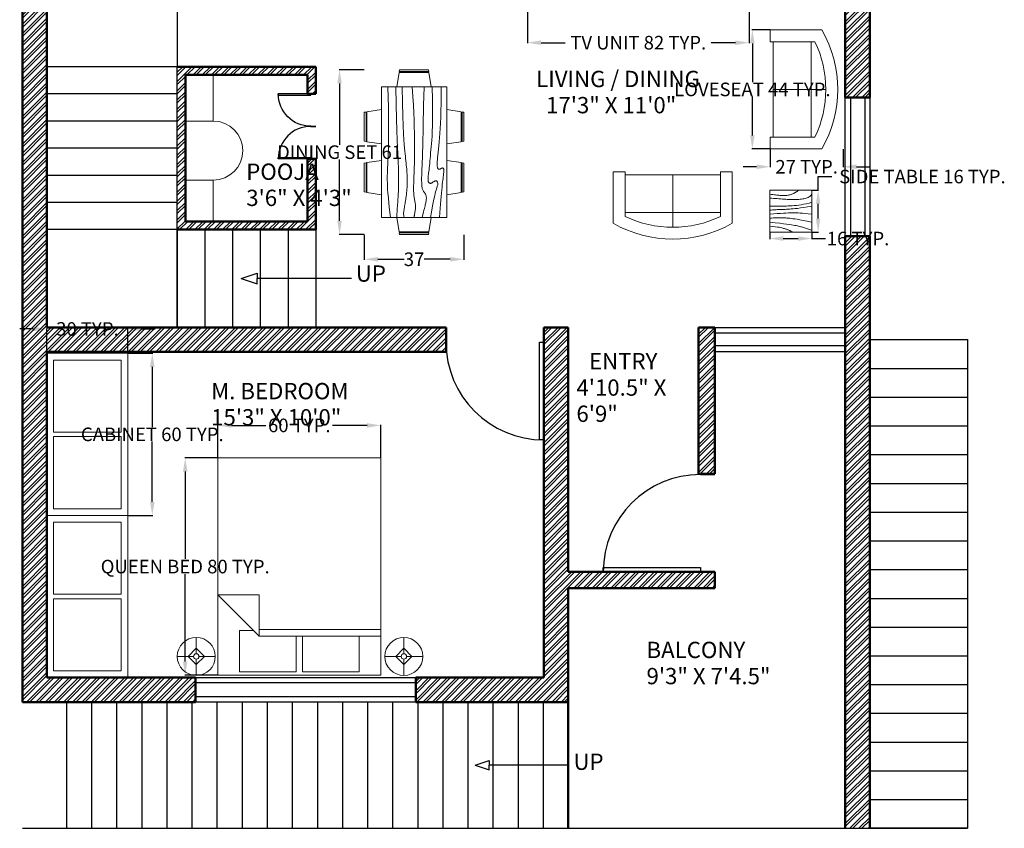
# Model space of a CAD drawing. Units: inches. Extents: x 0 to 822, y 0 to 962.
# Tile 1 of 3: x 23 to 385, y 501 to 799. Entities that reach past the tile are written whole.
import ezdxf

# ---------------------------------------------------------------- set-up
doc = ezdxf.new("R2010")
doc.units = ezdxf.units.IN
doc.header["$MEASUREMENT"] = 0
for name, color, linetype, lineweight in [('A-ANNO-DIMS', 2, 'Continuous', 18), ('A-ANNO-TEXT', 7, 'Continuous', 25), ('A-AREA-IDEN', 7, 'Continuous', 25), ('A-DOOR', 4, 'Continuous', 25), ('A-FLOR-CASE', 5, 'Continuous', 18), ('A-FLOR-STRS', 3, 'Continuous', 25), ('A-FURN', 9, 'Continuous', 18), ('A-GLAZ', 4, 'Continuous', 25), ('A-WALL', 7, 'Continuous', 50), ('A-WALL-PATT', 8, 'Continuous', 13)]:
    doc.layers.add(name, color=color, linetype=linetype, lineweight=lineweight)
doc.styles.get("Standard").update_dxf_attribs({"font": 'arial.ttf'})
doc.dimstyles.get("Standard").update_dxf_attribs({"dimtxt": 5, "dimasz": 5, "dimexe": 0.18, "dimexo": 0.0625, "dimgap": 0.09, "dimtad": 0, "dimtih": 1, "dimtoh": 1, "dimdec": 1, "dimzin": 0, "dimdsep": 46, "dimlunit": 4, "dimtxsty": 'Standard', "dimcen": 0.09, "dimadec": 0, "dimazin": 0, "dimtfac": 1, "dimtdec": 1, "dimtofl": 0, "dimtmove": 0, "dimatfit": 3, "dimfxl": 1, "dimtolj": 1, "dimtzin": 0, "dimarcsym": 0})

# ---------------------------------------------------------------- blocks, each defined once
blk = doc.blocks.new('*U2')
for p, q in [((0, 0), (0, -6)), ((40, 0), (40, -6))]:
    blk.add_line(p, q)
blk.add_lwpolyline([(0, 0), (0, 40), (1.75, 40), (1.75, 0)], close=True)
blk.add_arc((0, 0), 40, 0, 90)
blk = doc.blocks.new('Sofa - Roundback Loveseat 5 ft.')
for p, q in [((0, -32.44198), (0, -5.99998)), ((-24, -33.99998), (-24, -11.46958)), ((-23.9998, -13.38178), (23.99986, -13.38178)), ((24.00004, -33.99998), (24.00004, -11.46958)), ((-24, -32.44198), (24.00004, -32.44198))]:
    blk.add_line(p, q)
for points in [[(-24, -33.99998), (-30, -33.99998), (-30, -7.99998)], [(30.00004, -7.99998), (30.00004, -33.99998), (24.00004, -33.99998)]]:
    blk.add_lwpolyline(points)
for centre, radius, start, end in [((0, -60.24998), 60.24998, 60.13715, 119.8628), ((0, -61.38438), 55.38444, 64.32083, 115.6792)]:
    blk.add_arc(centre, radius, start, end)
blk = doc.blocks.new('Dining Set - 36 x 72 in.')
for p, q in [((-22, 27.5), (-22.1562, 26.50042)), ((-22, 27.5), (-6, 27.5)), ((-5.8437, 26.49966), (-6, 27.5)), ((6, 27.5), (5.8438, 26.50042)), ((6, 27.5), (22, 27.5)), ((22.1563, 26.49966), (22, 27.5)), ((-22.2343, 26.00059), (-23.4847, 17.99762)), ((-22.2304, 26), (-5.7608, 26)), ((-5.8416, 26.5), (-22.1534, 26.5)), ((-4.5152, 17.99762), (-5.7655, 25.99926)), ((5.7657, 26.00059), (4.5153, 17.99762)), ((5.7696, 26), (22.2392, 26)), ((22.1584, 26.5), (5.8466, 26.5)), ((23.4848, 17.99762), (22.2345, 25.99926)), ((36, 18), (-36, 18)), ((-36, 18), (-36, -18)), ((36, -18), (36, 18)), ((-45.5, 8), (-44.5004, 8.15617)), ((-45.5, 8), (-45.5, -8)), ((-44.5, -8.15843), (-44.5, 8.15338)), ((-44.0006, 8.23428), (-35.9976, 9.48474)), ((-44, 8.23041), (-44, -8.23915)), ((44.0006, 8.23428), (35.9976, 9.48474)), ((44, 8.23041), (44, -8.23915)), ((44.5, -8.15843), (44.5, 8.15338)), ((45.5, 8), (44.5005, 8.15617)), ((45.5, 8), (45.5, -8)), ((-44.4997, -8.15631), (-45.5, -8)), ((-35.9976, -9.48476), (-43.9993, -8.2345)), ((35.9976, -9.48476), (43.9993, -8.2345)), ((44.4997, -8.15631), (45.5, -8)), ((-36, -18), (36, -18)), ((-22.2343, -26.0006), (-23.4847, -17.99762)), ((-4.5152, -17.99762), (-5.7655, -25.99928)), ((5.7657, -26.0006), (4.5153, -17.99762)), ((23.4848, -17.99762), (22.2345, -25.99928)), ((-22.2304, -26), (-5.7608, -26)), ((-22, -27.5), (-22.1562, -26.50044)), ((-5.8416, -26.5), (-22.1534, -26.5)), ((-5.8437, -26.49967), (-6, -27.5)), ((5.7696, -26), (22.2392, -26)), ((6, -27.5), (5.8438, -26.50044)), ((22.1584, -26.5), (5.8466, -26.5)), ((22.1563, -26.49967), (22, -27.5)), ((-22, -27.5), (-6, -27.5)), ((6, -27.5), (22, -27.5))]:
    blk.add_line(p, q)
for points in [[(-36, 15), (-31.1772, 14.97754), (-26.8079, 14.91406), (-22.8538, 14.81543), (-19.276, 14.6875), (-16.0362, 14.53613), (-13.0957, 14.36718), (-10.4159, 14.18652), (-7.9583, 14), (-5.6904, 13.81315), (-3.6035, 13.63021), (-1.6954, 13.45508), (0.0365, 13.29166), (1.5945, 13.14388), (2.9811, 13.01562), (4.1988, 12.9108), (5.25, 12.83333), (6.1393, 12.78613), (6.8802, 12.76823), (7.4883, 12.77767), (7.9792, 12.8125), (8.3685, 12.87077), (8.6719, 12.95052), (8.9049, 13.0498), (9.0833, 13.16666), (9.2205, 13.29899), (9.3216, 13.44401), (9.3895, 13.59879), (9.4271, 13.76041), (9.4373, 13.92594), (9.4232, 14.09245), (9.3875, 14.257), (9.3333, 14.41666), (9.2638, 14.56917), (9.1836, 14.71484), (9.0975, 14.85465), (9.0104, 14.98958), (8.9272, 15.1206), (8.8529, 15.2487), (8.7922, 15.37483), (8.75, 15.5), (8.7305, 15.62467), (8.7344, 15.74739), (8.7617, 15.86621), (8.8125, 15.97916), (8.8867, 16.08431), (8.9844, 16.17968), (9.1055, 16.26334), (9.25, 16.33333), (9.4189, 16.38802), (9.6172, 16.42708), (9.8506, 16.45052), (10.125, 16.45833), (10.4463, 16.45052), (10.8203, 16.42708), (11.2529, 16.38802), (11.75, 16.33333), (12.3184, 16.26318), (12.9694, 16.17838), (13.7151, 16.07991), (14.5677, 15.96875), (15.5395, 15.84586), (16.6426, 15.71224), (17.8893, 15.56884), (19.2917, 15.41666), (20.859, 15.25667), (22.5879, 15.08984), (24.4721, 14.91715), (26.5052, 14.73958), (28.6809, 14.5581), (30.9929, 14.3737), (33.4347, 14.18733), (36, 14)], [(-36, 10), (-28.9766, 10.14274), (-23.1725, 10.20442), (-18.4241, 10.19775), (-14.5677, 10.13541), (-11.4399, 10.03011), (-8.877, 9.89453), (-6.7154, 9.74137), (-4.7917, 9.58333), (-2.9698, 9.43082), (-1.2246, 9.28515), (0.4415, 9.14534), (2.026, 9.01041), (3.5266, 8.87939), (4.9408, 8.7513), (6.266, 8.62516), (7.5, 8.5), (8.6411, 8.37549), (9.6914, 8.2539), (10.6538, 8.13818), (11.5312, 8.03125), (12.3267, 7.93603), (13.043, 7.85547), (13.6831, 7.79248), (14.25, 7.75), (14.7471, 7.7303), (15.1797, 7.73307), (15.5537, 7.75732), (15.875, 7.80208), (16.1494, 7.86637), (16.3828, 7.94922), (16.5811, 8.04964), (16.75, 8.16666), (16.8944, 8.29915), (17.0143, 8.44531), (17.1089, 8.60319), (17.1771, 8.77083), (17.218, 8.94629), (17.2305, 9.1276), (17.2137, 9.31282), (17.1667, 9.5), (17.0895, 9.6875), (16.987, 9.875), (16.8649, 10.0625), (16.7292, 10.25), (16.5856, 10.4375), (16.4401, 10.625), (16.2985, 10.8125), (16.1667, 11), (16.05, 11.18733), (15.9518, 11.3737), (15.8752, 11.5581), (15.8229, 11.73958), (15.798, 11.91715), (15.8034, 12.08984), (15.842, 12.25667), (15.9167, 12.41666), (16.0295, 12.56836), (16.1784, 12.70833), (16.3605, 12.83268), (16.5729, 12.9375), (16.8127, 13.01888), (17.0768, 13.07291), (17.3625, 13.0957), (17.6667, 13.08333), (17.9894, 13.03312), (18.3418, 12.94726), (18.7382, 12.82918), (19.1927, 12.68229), (19.7195, 12.51001), (20.3327, 12.31575), (21.0465, 12.10294), (21.875, 11.875), (22.8357, 11.63354), (23.959, 11.37304), (25.2786, 11.08618), (26.8282, 10.76562), (28.6414, 10.40405), (30.752, 9.99414), (33.1936, 9.52856), (36, 9)], [(-36, 5.5), (-30.7157, 5.3348), (-26.069, 5.20963), (-21.9946, 5.11767), (-18.4271, 5.05208), (-15.3009, 5.00602), (-12.5508, 4.97265), (-10.1112, 4.94515), (-7.9167, 4.91666), (-5.909, 4.88167), (-4.0586, 4.83984), (-2.3429, 4.79215), (-0.7396, 4.73958), (0.7739, 4.6831), (2.22, 4.6237), (3.6213, 4.56233), (5, 4.5), (6.373, 4.43782), (7.7344, 4.3776), (9.0723, 4.32129), (10.375, 4.27083), (11.6309, 4.22819), (12.8281, 4.19531), (13.9551, 4.17415), (15, 4.16666), (15.954, 4.17448), (16.819, 4.19791), (17.6001, 4.23698), (18.3021, 4.29166), (18.9299, 4.36198), (19.4883, 4.44791), (19.9823, 4.54948), (20.4167, 4.66666), (20.7969, 4.79899), (21.1302, 4.94401), (21.4245, 5.09879), (21.6875, 5.26041), (21.9271, 5.42594), (22.1511, 5.59245), (22.3672, 5.757), (22.5834, 5.91666), (22.8065, 6.06868), (23.0404, 6.21093), (23.2879, 6.34147), (23.5521, 6.45833), (23.8358, 6.55957), (24.142, 6.64323), (24.4735, 6.70735), (24.8334, 6.75), (25.2235, 6.76969), (25.642, 6.76692), (26.0858, 6.74267), (26.5521, 6.69791), (27.0379, 6.63362), (27.5404, 6.55078), (28.0565, 6.45036), (28.5834, 6.33333), (29.1242, 6.19987), (29.7071, 6.04687), (30.3661, 5.87044), (31.1354, 5.66666), (32.0493, 5.43164), (33.142, 5.16146), (34.4475, 4.85221), (36, 4.5)], [(-36, -1), (-30.7915, -0.6591), (-26.0195, -0.38216), (-21.6519, -0.16284), (-17.6563, 0.00521), (-14.0005, 0.12833), (-10.6523, 0.21289), (-7.5796, 0.26522), (-4.75, 0.29166), (-2.134, 0.29793), (0.2878, 0.28711), (2.5317, 0.26163), (4.6146, 0.22396), (6.5529, 0.17651), (8.3633, 0.12174), (10.0623, 0.06209), (11.6667, 0), (13.1899, -0.06201), (14.6341, -0.1211), (15.9982, -0.17432), (17.2813, -0.21875), (18.4823, -0.25147), (19.6003, -0.26953), (20.6343, -0.27002), (21.5834, -0.25), (22.4481, -0.20768), (23.2357, -0.14584), (23.9549, -0.06836), (24.6146, 0.02083), (25.2235, 0.11784), (25.7904, 0.21875), (26.3241, 0.31966), (26.8334, 0.41666), (27.3265, 0.50618), (27.8099, 0.58593), (28.2894, 0.65397), (28.7709, 0.70833), (29.2601, 0.74707), (29.763, 0.76823), (30.2855, 0.76985), (30.8334, 0.75), (31.4088, 0.70784), (31.9994, 0.64713), (32.589, 0.57275), (33.1615, 0.48958), (33.7008, 0.4025), (34.1908, 0.3164), (34.6153, 0.23616), (34.9584, 0.16666), (35.2099, 0.11165), (35.3848, 0.07031), (35.504, 0.04069), (35.5886, 0.02083), (35.6594, 0.00879), (35.7377, 0.0026), (35.8442, 0.00032), (36, 0)], [(-36, -6.5), (-27.1843, -6.31267), (-20.084, -6.1263), (-14.469, -5.9419), (-10.1094, -5.76042), (-6.7752, -5.58285), (-4.2363, -5.41016), (-2.2629, -5.24333), (-0.625, -5.08334), (0.8708, -4.93099), (2.2715, -4.78646), (3.5872, -4.64974), (4.8281, -4.52084), (6.0046, -4.39974), (7.127, -4.28646), (8.2053, -4.18099), (9.25, -4.08334), (10.2705, -3.99382), (11.2734, -3.91407), (12.2647, -3.84603), (13.25, -3.79167), (14.2354, -3.75293), (15.2266, -3.73177), (16.2295, -3.73015), (17.25, -3.75), (18.2912, -3.79248), (19.3451, -3.85547), (20.4009, -3.93604), (21.4479, -4.03125), (22.4754, -4.13819), (23.4727, -4.25391), (24.4289, -4.37549), (25.3334, -4.5), (26.1785, -4.62492), (26.9694, -4.74935), (27.7145, -4.87281), (28.4219, -4.99479), (29.1, -5.11483), (29.7572, -5.23242), (30.4016, -5.34709), (31.0417, -5.45834), (31.6837, -5.56437), (32.3262, -5.65821), (32.9658, -5.73153), (33.599, -5.77604), (34.2224, -5.78345), (34.8327, -5.74545), (35.4264, -5.65373), (36, -5.5)], [(-36, -10), (-26.4022, -9.81299), (-18.4675, -9.62891), (-11.9839, -9.45069), (-6.7396, -9.28125), (-2.5226, -9.12354), (0.8789, -8.98047), (3.6769, -8.85498), (6.0833, -8.75), (8.2767, -8.66765), (10.3021, -8.60677), (12.1712, -8.56543), (13.8958, -8.54167), (15.4876, -8.53353), (16.9583, -8.53907), (18.3197, -8.55632), (19.5834, -8.58334), (20.7616, -8.61841), (21.8685, -8.66081), (22.9188, -8.71004), (23.9271, -8.76563), (24.9081, -8.82707), (25.8763, -8.89388), (26.8465, -8.96558), (27.8334, -9.04167), (28.8474, -9.12118), (29.8828, -9.20117), (30.93, -9.27824), (31.9792, -9.34896), (33.0205, -9.40991), (34.0443, -9.45768), (35.0407, -9.48885), (36, -9.5)], [(-36, -14.5), (-30.0881, -14.33513), (-25.0332, -14.21224), (-20.7312, -14.12647), (-17.0781, -14.07292), (-13.97, -14.04671), (-11.3027, -14.04297), (-8.9724, -14.05681), (-6.875, -14.08334), (-4.9224, -14.11833), (-3.0905, -14.16016), (-1.3709, -14.20785), (0.2448, -14.26042), (1.7647, -14.3169), (3.1973, -14.3763), (4.5507, -14.43767), (5.8333, -14.5), (7.0554, -14.5621), (8.235, -14.62175), (9.3922, -14.67652), (10.5469, -14.72396), (11.7192, -14.76164), (12.929, -14.78711), (14.1965, -14.79794), (15.5417, -14.79167), (16.9933, -14.76424), (18.6152, -14.70508), (20.4804, -14.60197), (22.6615, -14.44271), (25.2312, -14.21509), (28.2624, -13.9069), (31.8277, -13.50594), (36, -13)]]:
    blk.add_lwpolyline(points)
blk = doc.blocks.new('Table - Square Woodgrain 42 x 42 in.')
blk.add_line((0, -42), (42, -42))
for points in [[(0, -4), (1.704, -4.2172), (3.2358, -4.4188), (4.615, -4.604), (5.8615, -4.7721), (6.9951, -4.9224), (8.0357, -5.0541), (9.0031, -5.1667), (9.9171, -5.2594), (10.7951, -5.3316), (11.6445, -5.3836), (12.4702, -5.4157), (13.277, -5.4283), (14.0698, -5.4217), (14.8535, -5.3964), (15.6331, -5.3526), (16.4133, -5.2908), (17.1986, -5.2103), (17.9913, -5.1062), (18.793, -4.9727), (19.6056, -4.8038), (20.4307, -4.5937), (21.2701, -4.3365), (22.1256, -4.0262), (22.9989, -3.6571), (23.888, -3.2272), (24.7756, -2.7516), (25.6408, -2.2491), (26.4624, -1.7387), (27.2195, -1.2395), (27.891, -0.7703), (28.456, -0.3501), (28.8934, 0.002)], [(0, -42), (0, 0), (42, 0), (42, -42)], [(0, -8), (1.8203, -8.1001), (3.6741, -8.2149), (5.5411, -8.3408), (7.4011, -8.4741), (9.2339, -8.6112), (11.0193, -8.7484), (12.7371, -8.8821), (14.3671, -9.0086), (15.8954, -9.1246), (17.3337, -9.2278), (18.6997, -9.3159), (20.0116, -9.387), (21.2871, -9.4389), (22.5442, -9.4696), (23.8008, -9.477), (25.0749, -9.459), (26.3791, -9.4137), (27.7049, -9.3403), (29.0383, -9.2382), (30.3655, -9.1068), (31.6728, -8.9455), (32.9461, -8.7535), (34.1717, -8.5304), (35.3358, -8.2756), (36.4268, -7.9863), (37.443, -7.6521), (38.3849, -7.2603), (39.253, -6.7986), (40.048, -6.2542), (40.7705, -5.6147), (41.421, -4.8674), (42, -4)], [(42, -12), (39.1784, -12.8621), (36.4519, -13.5654), (33.8246, -14.1294), (31.3004, -14.5731), (28.8832, -14.9161), (26.577, -15.1775), (24.3858, -15.3768), (22.3136, -15.5332), (20.3622, -15.6632), (18.5254, -15.7718), (16.7947, -15.8612), (15.1618, -15.9338), (13.6183, -15.9916), (12.1558, -16.0369), (10.7659, -16.0718), (9.4403, -16.0987), (8.1703, -16.1191), (6.9461, -16.1325), (5.7577, -16.1377), (4.595, -16.1335), (3.4479, -16.1188), (2.3064, -16.0924), (1.1604, -16.0532), (0, -16)], [(42, -16), (37.6529, -16.7365), (33.8802, -17.329), (30.6179, -17.7961), (27.8015, -18.1561), (25.3668, -18.4275), (23.2497, -18.6288), (21.3859, -18.7785), (19.7111, -18.8949), (18.1693, -18.9939), (16.7375, -19.0795), (15.401, -19.1534), (14.1449, -19.217), (12.9544, -19.2717), (11.8148, -19.3191), (10.7113, -19.3606), (9.6291, -19.3976), (8.5534, -19.4323), (7.47, -19.4689), (6.3643, -19.5122), (5.222, -19.5672), (4.0288, -19.6386), (2.7703, -19.7313), (1.4321, -19.8501), (0, -20)], [(0, -24), (3.9243, -23.6805), (7.4766, -23.4138), (10.6891, -23.1954), (13.5943, -23.0205), (16.2247, -22.8847), (18.6125, -22.7832), (20.7903, -22.7116), (22.7903, -22.6651), (24.6563, -22.642), (26.4764, -22.6507), (28.35, -22.7024), (30.3766, -22.8084), (32.6555, -22.98), (35.2861, -23.2283), (38.3678, -23.5645), (42, -24)], [(42, -32), (37.392, -31.017), (33.4585, -30.2231), (30.1291, -29.5949), (27.3334, -29.109), (25.0009, -28.742), (23.0612, -28.4707), (21.4439, -28.2716), (20.0786, -28.1215), (18.8998, -28.0002), (17.8609, -27.9014), (16.9206, -27.8219), (16.0371, -27.7588), (15.1691, -27.709), (14.2748, -27.6693), (13.3128, -27.6368), (12.2415, -27.6083), (11.0295, -27.5824), (9.6867, -27.5643), (8.233, -27.5608), (6.6884, -27.5787), (5.0728, -27.6248), (3.4062, -27.7058), (1.7086, -27.8286), (0, -28)], [(0, -32), (5.4026, -32.5358), (9.9494, -33.019), (13.7424, -33.4553), (16.8834, -33.8505), (19.4743, -34.2106), (21.6171, -34.5413), (23.4136, -34.8486), (24.9657, -35.1382), (26.3614, -35.4156), (27.6332, -35.6841), (28.7995, -35.9467), (29.8788, -36.2064), (30.8897, -36.4661), (31.8507, -36.7288), (32.7802, -36.9973), (33.6968, -37.2747), (34.6175, -37.5635), (35.5531, -37.8651), (36.5128, -38.1805), (37.506, -38.5108), (38.5421, -38.8568), (39.6302, -39.2197), (40.7797, -39.6004), (42, -40)], [(0, -36), (3.0098, -36.2857), (5.5354, -36.5643), (7.6368, -36.8359), (9.374, -37.1009), (10.807, -37.3597), (11.9957, -37.6126), (13.0002, -37.8599), (13.8804, -38.102), (14.6874, -38.3393), (15.4365, -38.5729), (16.1338, -38.8041), (16.7858, -39.0341), (17.3987, -39.264), (17.9787, -39.4952), (18.5322, -39.7288), (19.0655, -39.9662), (19.5832, -40.2081), (20.0842, -40.4544), (20.5657, -40.7046), (21.0249, -40.9581), (21.459, -41.2144), (21.8653, -41.4731), (22.2409, -41.7335), (22.5831, -41.9951)]]:
    blk.add_lwpolyline(points)
blk = doc.blocks.new('Bed - Queen')
for p, q in [((0, -80.00003), (0, 0)), ((0, 0), (59.99999, 0)), ((59.99999, 0), (59.99999, -80.00003)), ((7.99999, -1.2), (28.79998, -1.2)), ((7.99999, -14.4), (7.99999, -1.2)), ((28.79998, -1.2), (28.79998, -14.4)), ((31.19999, -1.2), (51.99999, -1.2)), ((31.19999, -14.4), (31.19999, -1.2)), ((51.99999, -1.2), (51.99999, -16.4)), ((0, -14.4), (44.8, -14.4)), ((59.99999, -29.6), (44.8, -14.4)), ((44.8, -14.4), (44.8, -29.6)), ((44.8, -16.8), (0, -16.8)), ((51.99999, -16.4), (46.79936, -16.4)), ((44.8, -29.6), (59.99999, -29.6)), ((59.99999, -80.00003), (0, -80.00003))]:
    blk.add_line(p, q)
blk = doc.blocks.new('Lamp - Table')
for p, q in [((0, 7), (0, 1)), ((-1, 0), (-7, 0)), ((0, 3), (-3, 0)), ((-3, 0), (0, -3)), ((3, 0), (0, 3)), ((0, -3), (3, 0)), ((1, 0), (7, 0)), ((0, -1), (0, -7))]:
    blk.add_line(p, q)
for radius in [7, 1]:
    blk.add_circle((0, 0), radius)
blk = doc.blocks.new('Wall Cabinet - 18 x 36 in front')
for p, q in [((17.5, -1.5), (17.5, -16.5)), ((18.5, -16.5), (18.5, -1.5))]:
    blk.add_line(p, q)
blk.add_lwpolyline([(0, -18), (0, 0), (36, 0), (36, -18)], close=True)
for points in [[(17.5, -16.5), (1.5, -16.5), (1.5, -1.5), (17.5, -1.5)], [(18.5, -1.5), (34.5, -1.5), (34.5, -16.5), (18.5, -16.5)]]:
    blk.add_lwpolyline(points)
blk = doc.blocks.new('STAIR-ARROW')
for p, q in [((0, 1.94), (5.97, 3.89)), ((5.97, 3.89), (5.97, 1.94)), ((0, 1.94), (5.97, 0)), ((40.68, 1.94), (5.97, 1.94)), ((5.97, 0), (5.97, 1.94))]:
    blk.add_line(p, q)
blk = doc.blocks.new('*D15')
at = {"layer": 'A-ANNO-DIMS', "color": 0, "lineweight": -2, "transparency": 16777216}
for p, q in [((95.61, 637.85), (83.49, 637.85)), ((83.67, 632.85), (83.67, 600.67)), ((83.67, 562.85), (83.67, 595.02)), ((95.61, 557.85), (83.49, 557.85))]:
    blk.add_line(p, q, dxfattribs=at)
at = {"layer": 'A-ANNO-DIMS', "color": 0, "transparency": 16777216}
for points in [[(82.84, 632.85), (84.5, 632.85), (83.67, 637.85)], [(82.84, 562.85), (84.5, 562.85), (83.67, 557.85)]]:
    blk.add_solid(points, dxfattribs=at)
at = {"layer": 'Defpoints', "color": 0, "transparency": 16777216}
for p in [(95.67, 637.85), (83.67, 557.85), (95.67, 557.85)]:
    blk.add_point(p, dxfattribs=at)
at = {"layer": 'A-ANNO-DIMS', "color": 0, "transparency": 16777216, "insert": (83.67, 597.85), "char_height": 5, "attachment_point": 5}
blk.add_mtext('\\A1;QUEEN BED 80 TYP.', dxfattribs=at)
blk = doc.blocks.new('*D16')
at = {"layer": 'A-ANNO-DIMS', "color": 0, "lineweight": -2, "transparency": 16777216}
for p, q in [((95.67, 637.91), (95.67, 650.03)), ((100.67, 649.85), (113.4, 649.85)), ((150.67, 649.85), (137.94, 649.85)), ((155.67, 637.91), (155.67, 650.03))]:
    blk.add_line(p, q, dxfattribs=at)
at = {"layer": 'A-ANNO-DIMS', "color": 0, "transparency": 16777216}
for points in [[(100.67, 650.68), (100.67, 649.01), (95.67, 649.85)], [(150.67, 650.68), (150.67, 649.01), (155.67, 649.85)]]:
    blk.add_solid(points, dxfattribs=at)
at = {"layer": 'Defpoints', "color": 0, "transparency": 16777216}
for p in [(95.67, 649.85), (95.67, 637.85), (155.67, 637.85)]:
    blk.add_point(p, dxfattribs=at)
at = {"layer": 'A-ANNO-DIMS', "color": 0, "transparency": 16777216, "insert": (125.67, 649.85), "char_height": 5, "attachment_point": 5}
blk.add_mtext('\\A1;60 TYP.', dxfattribs=at)
blk = doc.blocks.new('*D23')
at = {"layer": 'A-ANNO-DIMS', "color": 0, "lineweight": -2, "transparency": 16777216}
for p, q in [((62.66, 676.41), (71.73, 676.41)), ((71.55, 671.41), (71.55, 649.22)), ((71.55, 621.68), (71.55, 643.87)), ((62.66, 616.68), (71.73, 616.68))]:
    blk.add_line(p, q, dxfattribs=at)
at = {"layer": 'A-ANNO-DIMS', "color": 0, "transparency": 16777216}
for points in [[(70.72, 671.41), (72.39, 671.41), (71.55, 676.41)], [(70.72, 621.68), (72.39, 621.68), (71.55, 616.68)]]:
    blk.add_solid(points, dxfattribs=at)
at = {"layer": 'Defpoints', "color": 0, "transparency": 16777216}
for p in [(62.59, 676.41), (62.59, 616.68), (71.55, 616.68)]:
    blk.add_point(p, dxfattribs=at)
at = {"layer": 'A-ANNO-DIMS', "color": 0, "transparency": 16777216, "insert": (71.55, 646.55), "char_height": 5, "attachment_point": 5}
blk.add_mtext('\\A1;CABINET 60 TYP.', dxfattribs=at)
blk = doc.blocks.new('*D24')
at = {"layer": 'A-ANNO-DIMS', "color": 0, "lineweight": -2, "transparency": 16777216}
for p, q in [((27.73, 685.37), (22.73, 685.37)), ((32.73, 676.48), (32.73, 685.55)), ((62.59, 676.48), (62.59, 685.55)), ((67.59, 685.37), (72.59, 685.37))]:
    blk.add_line(p, q, dxfattribs=at)
at = {"layer": 'A-ANNO-DIMS', "color": 0, "transparency": 16777216}
for points in [[(27.73, 686.21), (27.73, 684.54), (32.73, 685.37)], [(67.59, 686.21), (67.59, 684.54), (62.59, 685.37)]]:
    blk.add_solid(points, dxfattribs=at)
at = {"layer": 'Defpoints', "color": 0, "transparency": 16777216}
for p in [(62.59, 685.37), (32.73, 676.41), (62.59, 676.41)]:
    blk.add_point(p, dxfattribs=at)
at = {"layer": 'A-ANNO-DIMS', "color": 0, "transparency": 16777216, "insert": (47.66, 685.37), "char_height": 5, "attachment_point": 5}
blk.add_mtext('\\A1;30 TYP.', dxfattribs=at)
blk = doc.blocks.new('*D25')
at = {"layer": 'A-ANNO-DIMS', "color": 0, "lineweight": -2, "transparency": 16777216}
for p, q in [((299.03, 795.53), (292.33, 795.53)), ((292.51, 790.53), (292.51, 776.28)), ((292.51, 756.68), (292.51, 770.93)), ((299.03, 751.68), (292.33, 751.68))]:
    blk.add_line(p, q, dxfattribs=at)
at = {"layer": 'A-ANNO-DIMS', "color": 0, "transparency": 16777216}
for points in [[(291.68, 790.53), (293.35, 790.53), (292.51, 795.53)], [(291.68, 756.68), (293.35, 756.68), (292.51, 751.68)]]:
    blk.add_solid(points, dxfattribs=at)
at = {"layer": 'Defpoints', "color": 0, "transparency": 16777216}
for p in [(299.09, 795.53), (292.51, 751.68), (299.09, 751.68)]:
    blk.add_point(p, dxfattribs=at)
at = {"layer": 'A-ANNO-DIMS', "color": 0, "transparency": 16777216, "insert": (292.51, 773.6), "char_height": 5, "attachment_point": 5}
blk.add_mtext('\\A1;LOVESEAT 44 TYP.', dxfattribs=at)
blk = doc.blocks.new('*D26')
at = {"layer": 'A-ANNO-DIMS', "color": 0, "lineweight": -2, "transparency": 16777216}
for p, q in [((299.09, 751.62), (299.09, 744.92)), ((325.89, 751.62), (325.89, 744.92)), ((294.09, 745.1), (289.09, 745.1)), ((330.89, 745.1), (335.89, 745.1))]:
    blk.add_line(p, q, dxfattribs=at)
at = {"layer": 'A-ANNO-DIMS', "color": 0, "transparency": 16777216}
for points in [[(294.09, 745.94), (294.09, 744.27), (299.09, 745.1)], [(330.89, 745.94), (330.89, 744.27), (325.89, 745.1)]]:
    blk.add_solid(points, dxfattribs=at)
at = {"layer": 'Defpoints', "color": 0, "transparency": 16777216}
for p in [(299.09, 751.68), (325.89, 751.68), (325.89, 745.1)]:
    blk.add_point(p, dxfattribs=at)
at = {"layer": 'A-ANNO-DIMS', "color": 0, "transparency": 16777216, "insert": (312.49, 745.1), "char_height": 5, "attachment_point": 5}
blk.add_mtext('\\A1;27 TYP.', dxfattribs=at)
blk = doc.blocks.new('*D27')
at = {"layer": 'A-ANNO-DIMS', "color": 0, "lineweight": -2, "transparency": 16777216}
for p, q in [((209.73, 802.98), (209.73, 790.63)), ((291.28, 802.98), (291.28, 790.63)), ((214.73, 790.81), (223.63, 790.81)), ((286.28, 790.81), (277.38, 790.81))]:
    blk.add_line(p, q, dxfattribs=at)
at = {"layer": 'A-ANNO-DIMS', "color": 0, "transparency": 16777216}
for points in [[(214.73, 791.64), (214.73, 789.97), (209.73, 790.81)], [(286.28, 791.64), (286.28, 789.97), (291.28, 790.81)]]:
    blk.add_solid(points, dxfattribs=at)
at = {"layer": 'Defpoints', "color": 0, "transparency": 16777216}
for p in [(209.73, 803.04), (291.28, 803.04), (291.28, 790.81)]:
    blk.add_point(p, dxfattribs=at)
at = {"layer": 'A-ANNO-DIMS', "color": 0, "transparency": 16777216, "insert": (250.5, 790.81), "char_height": 5, "attachment_point": 5}
blk.add_mtext('\\A1;TV UNIT 82 TYP.', dxfattribs=at)
blk = doc.blocks.new('*D29')
at = {"layer": 'A-ANNO-DIMS', "color": 0, "lineweight": -2, "transparency": 16777216}
for p, q in [((316.74, 736.5), (316.74, 741.5)), ((316.74, 741.5), (321.74, 741.5)), ((314.47, 736.5), (316.92, 736.5)), ((316.74, 726), (316.74, 731.5)), ((314.47, 721), (316.92, 721))]:
    blk.add_line(p, q, dxfattribs=at)
at = {"layer": 'A-ANNO-DIMS', "color": 0, "transparency": 16777216}
for points in [[(315.9, 731.5), (317.57, 731.5), (316.74, 736.5)], [(315.9, 726), (317.57, 726), (316.74, 721)]]:
    blk.add_solid(points, dxfattribs=at)
at = {"layer": 'Defpoints', "color": 0, "transparency": 16777216}
for p in [(314.41, 736.5), (316.74, 736.5), (314.41, 721)]:
    blk.add_point(p, dxfattribs=at)
at = {"layer": 'A-ANNO-DIMS', "color": 0, "transparency": 16777216, "insert": (355.14, 741.5), "char_height": 5, "attachment_point": 5}
blk.add_mtext('\\A1;SIDE TABLE 16 TYP.', dxfattribs=at)
blk = doc.blocks.new('*D30')
at = {"layer": 'A-ANNO-DIMS', "color": 0, "lineweight": -2, "transparency": 16777216}
for p, q in [((298.91, 720.93), (298.91, 718.49)), ((303.91, 718.67), (309.41, 718.67)), ((314.41, 720.93), (314.41, 718.49)), ((314.41, 718.67), (319.41, 718.67))]:
    blk.add_line(p, q, dxfattribs=at)
at = {"layer": 'A-ANNO-DIMS', "color": 0, "transparency": 16777216}
for points in [[(303.91, 719.5), (303.91, 717.84), (298.91, 718.67)], [(309.41, 719.5), (309.41, 717.84), (314.41, 718.67)]]:
    blk.add_solid(points, dxfattribs=at)
at = {"layer": 'Defpoints', "color": 0, "transparency": 16777216}
for p in [(298.91, 721), (314.41, 721), (314.41, 718.67)]:
    blk.add_point(p, dxfattribs=at)
at = {"layer": 'A-ANNO-DIMS', "color": 0, "transparency": 16777216, "insert": (331.43, 718.67), "char_height": 5, "attachment_point": 5}
blk.add_mtext('\\A1;16 TYP.', dxfattribs=at)
blk = doc.blocks.new('*D35')
at = {"layer": 'A-ANNO-DIMS', "color": 0, "lineweight": -2, "transparency": 16777216}
for p, q in [((149.55, 780.83), (140.33, 780.83)), ((140.51, 775.83), (140.51, 753.16)), ((140.51, 725.14), (140.51, 747.81)), ((149.55, 720.14), (140.33, 720.14))]:
    blk.add_line(p, q, dxfattribs=at)
at = {"layer": 'A-ANNO-DIMS', "color": 0, "transparency": 16777216}
for points in [[(139.67, 775.83), (141.34, 775.83), (140.51, 780.83)], [(139.67, 725.14), (141.34, 725.14), (140.51, 720.14)]]:
    blk.add_solid(points, dxfattribs=at)
at = {"layer": 'Defpoints', "color": 0, "transparency": 16777216}
for p in [(149.61, 780.83), (140.51, 720.14), (149.61, 720.14)]:
    blk.add_point(p, dxfattribs=at)
at = {"layer": 'A-ANNO-DIMS', "color": 0, "transparency": 16777216, "insert": (140.51, 750.49), "char_height": 5, "attachment_point": 5}
blk.add_mtext('\\A1;DINING SET 61', dxfattribs=at)
blk = doc.blocks.new('*D36')
at = {"layer": 'A-ANNO-DIMS', "color": 0, "lineweight": -2, "transparency": 16777216}
for p, q in [((149.61, 720.08), (149.61, 710.86)), ((186.29, 720.08), (186.29, 710.86)), ((154.61, 711.04), (164.28, 711.04)), ((181.29, 711.04), (171.62, 711.04))]:
    blk.add_line(p, q, dxfattribs=at)
at = {"layer": 'A-ANNO-DIMS', "color": 0, "transparency": 16777216}
for points in [[(154.61, 711.87), (154.61, 710.2), (149.61, 711.04)], [(181.29, 711.87), (181.29, 710.2), (186.29, 711.04)]]:
    blk.add_solid(points, dxfattribs=at)
at = {"layer": 'Defpoints', "color": 0, "transparency": 16777216}
for p in [(149.61, 720.14), (186.29, 720.14), (186.29, 711.04)]:
    blk.add_point(p, dxfattribs=at)
at = {"layer": 'A-ANNO-DIMS', "color": 0, "transparency": 16777216, "insert": (167.95, 711.04), "char_height": 5, "attachment_point": 5}
blk.add_mtext('\\A1;37', dxfattribs=at)

msp = doc.modelspace()

# ---------------------------------------------------------------- hatches: boundary and pattern name
at = {"layer": 'A-WALL-PATT', "transparency": 33554641}
h = msp.add_hatch(dxfattribs=at)
h.set_pattern_fill('ANSI32', color=256, scale=6.4)
h.paths.add_polyline_path([(149.73, 826.95), (23.73, 826.95), (23.73, 547.95), (87.48, 547.95), (87.48, 556.95), (32.73, 556.95), (32.73, 676.95), (179.73, 676.95), (179.73, 685.95), (32.73, 685.95), (32.73, 817.95), (149.73, 817.95)])
h.paths.add_polyline_path([(224.73, 685.95), (215.73, 685.95), (215.73, 556.95), (168.56, 556.95), (168.56, 547.95), (224.73, 547.95), (224.73, 589.95), (278.73, 589.95), (278.73, 595.95), (224.73, 595.95)])
h.paths.add_polyline_path([(278.73, 685.95), (272.73, 685.95), (272.73, 631.95), (278.73, 631.95)])
h.paths.add_polyline_path([(335.73, 719.52), (326.73, 719.52), (326.73, 676.95), (326.73, 589.95), (326.73, 501.45), (335.73, 501.45)])
h.paths.add_polyline_path([(335.73, 846.75), (326.73, 846.75), (326.73, 826.95), (209.73, 826.95), (209.73, 817.95), (326.73, 817.95), (326.73, 770.62), (335.73, 770.62)])
h.paths.add_polyline_path([(218.73, 952.95), (326.73, 952.95), (326.73, 927.05), (335.73, 927.05), (335.73, 961.95), (209.73, 961.95), (209.73, 952.95), (209.73, 862.95), (218.73, 862.95)])
h.paths.add_polyline_path([(149.73, 952.95), (170.53, 952.95), (170.53, 961.95), (23.73, 961.95), (23.73, 878.05), (32.73, 878.05), (32.73, 952.95), (140.73, 952.95), (140.73, 862.95), (185.73, 862.95), (185.73, 868.95), (149.73, 868.95)])
h = msp.add_hatch(dxfattribs=at)
h.set_pattern_fill('ANSI32', color=256, scale=6.4)
h.paths.add_polyline_path([(131.73, 724.95), (131.73, 748.01), (128.73, 748.01), (128.73, 724.95), (83.73, 724.95), (83.73, 740.23), (83.73, 778.95), (128.73, 778.95), (128.73, 772.01), (131.73, 772.01), (131.73, 778.95), (131.73, 781.95), (80.73, 781.95), (80.73, 721.95), (131.73, 721.95)])

# ---------------------------------------------------------------- linework, layer by layer
at = {"layer": 'A-FLOR-STRS'}
for p, q in [((80.73, 817.95), (80.73, 781.95)), ((80.73, 781.95), (32.73, 781.95)), ((80.73, 721.95), (80.73, 781.95)), ((80.73, 771.95), (32.73, 771.95)), ((80.73, 761.95), (32.73, 761.95)), ((80.73, 751.95), (32.73, 751.95)), ((80.73, 741.95), (32.73, 741.95)), ((80.73, 731.95), (32.73, 731.95)), ((80.73, 721.95), (32.73, 721.95)), ((80.73, 721.95), (32.73, 721.95)), ((80.73, 685.95), (80.73, 721.95)), ((80.73, 721.95), (80.73, 685.95)), ((90.93, 721.95), (90.93, 685.95)), ((101.13, 721.95), (101.13, 685.95)), ((111.33, 721.95), (111.33, 685.95)), ((121.53, 721.95), (121.53, 685.95)), ((131.73, 721.95), (131.73, 685.95)), ((335.73, 681.45), (371.73, 681.45)), ((371.73, 681.45), (371.73, 501.45)), ((335.73, 670.86), (371.73, 670.86)), ((335.73, 660.27), (371.73, 660.27)), ((335.73, 649.68), (371.73, 649.68)), ((335.73, 639.09), (371.73, 639.09)), ((335.73, 628.5), (371.73, 628.5)), ((335.73, 617.92), (371.73, 617.92)), ((335.73, 607.33), (371.73, 607.33)), ((335.73, 596.74), (371.73, 596.74)), ((335.73, 586.15), (371.73, 586.15)), ((335.73, 575.56), (371.73, 575.56)), ((335.73, 564.97), (371.73, 564.97)), ((335.73, 554.39), (371.73, 554.39)), ((39.93, 547.95), (39.93, 501.45)), ((49.17, 547.95), (49.17, 501.45)), ((58.41, 547.95), (58.41, 501.45)), ((67.65, 547.95), (67.65, 501.45)), ((76.89, 547.95), (76.89, 501.45)), ((86.13, 547.95), (86.13, 501.45)), ((95.37, 547.95), (95.37, 501.45)), ((104.61, 547.95), (104.61, 501.45)), ((113.85, 547.95), (113.85, 501.45)), ((123.09, 547.95), (123.09, 501.45)), ((132.33, 547.95), (132.33, 501.45)), ((141.57, 547.95), (141.57, 501.45)), ((150.81, 547.95), (150.81, 501.45)), ((160.05, 547.95), (160.05, 501.45)), ((169.29, 547.95), (169.29, 501.45)), ((178.53, 547.95), (178.53, 501.45)), ((187.77, 547.95), (187.77, 501.45)), ((197.01, 547.95), (197.01, 501.45)), ((206.25, 547.95), (206.25, 501.45)), ((215.49, 547.95), (215.49, 501.45)), ((224.73, 547.95), (224.73, 501.45)), ((335.73, 543.8), (371.73, 543.8)), ((335.73, 533.21), (371.73, 533.21)), ((190.45, 524.7), (195.65, 526.46)), ((195.65, 526.46), (195.65, 524.7)), ((190.45, 524.7), (195.65, 522.93)), ((224.73, 524.7), (195.65, 524.7)), ((195.65, 522.93), (195.65, 524.7)), ((335.73, 522.62), (371.73, 522.62)), ((335.73, 512.03), (371.73, 512.03)), ((23.73, 501.45), (335.73, 501.45)), ((371.73, 501.45), (335.73, 501.45)), ((335.73, 501.45), (371.73, 501.45))]:
    msp.add_line(p, q, dxfattribs=at)
at = {"layer": 'A-FURN'}
for p, q in [((94, 761.95), (94, 778.95)), ((83.73, 761.95), (94, 761.95)), ((83.73, 740.23), (94, 740.23)), ((94, 740.23), (94, 724.95))]:
    msp.add_line(p, q, dxfattribs=at)
msp.add_arc((94, 751.09), 10.86, 270, 90, dxfattribs=at)
at = {"layer": 'A-GLAZ'}
for points in [[(335.73, 719.52), (326.73, 719.52), (326.73, 770.62), (335.73, 770.62)], [(328.74, 770.62), (333.93, 770.62), (333.93, 719.52), (328.74, 719.52)], [(278.73, 685.95), (326.73, 685.95), (326.73, 676.95), (278.73, 676.95)], [(278.73, 683.91), (326.73, 683.91), (326.73, 679.21), (278.73, 679.21)], [(87.48, 556.95), (168.56, 556.95), (168.56, 547.95), (87.48, 547.95)], [(87.48, 555.12), (168.56, 555.12), (168.56, 549.91), (87.48, 549.91)]]:
    msp.add_lwpolyline(points, close=True, dxfattribs=at)
at = {"layer": 'A-WALL'}
for p, q in [((335.73, 846.75), (335.73, 770.62)), ((23.73, 826.95), (23.73, 547.95)), ((32.73, 817.95), (32.73, 685.95)), ((326.73, 817.95), (326.73, 770.62)), ((80.73, 781.95), (131.73, 781.95)), ((131.73, 781.95), (131.73, 778.95)), ((83.73, 724.95), (83.73, 778.95)), ((83.73, 778.95), (128.73, 778.95)), ((128.73, 778.95), (128.73, 772.01)), ((131.73, 778.95), (131.73, 772.01)), ((128.73, 772.01), (131.73, 772.01)), ((326.73, 770.62), (335.73, 770.62)), ((131.73, 748.01), (128.73, 748.01)), ((128.73, 748.01), (128.73, 724.95)), ((131.73, 748.01), (131.73, 724.95)), ((80.73, 721.95), (131.73, 721.95)), ((128.73, 724.95), (83.73, 724.95)), ((131.73, 721.95), (131.73, 724.95)), ((326.73, 719.52), (335.73, 719.52)), ((326.73, 719.52), (326.73, 676.95)), ((335.73, 719.52), (335.73, 501.45)), ((32.73, 685.95), (179.73, 685.95)), ((179.73, 676.95), (179.73, 685.95)), ((215.73, 685.95), (215.73, 556.95)), ((215.73, 685.95), (224.73, 685.95)), ((224.73, 685.95), (224.73, 595.95)), ((272.73, 685.95), (272.73, 631.95)), ((272.73, 685.95), (278.73, 685.95)), ((278.73, 685.95), (278.73, 631.95)), ((32.73, 676.95), (179.73, 676.95)), ((32.73, 676.95), (32.73, 556.95)), ((326.73, 676.95), (326.73, 589.95)), ((272.73, 631.95), (278.73, 631.95)), ((224.73, 595.95), (278.73, 595.95)), ((278.73, 595.95), (278.73, 589.95)), ((224.73, 589.95), (278.73, 589.95)), ((224.73, 589.95), (224.73, 501.45)), ((326.73, 589.95), (326.73, 501.45)), ((32.73, 556.95), (87.48, 556.95)), ((87.48, 556.95), (87.48, 547.95)), ((168.56, 556.95), (168.56, 547.95)), ((168.56, 556.95), (215.73, 556.95)), ((23.73, 547.95), (87.48, 547.95)), ((168.56, 547.95), (224.73, 547.95))]:
    msp.add_line(p, q, dxfattribs=at)

# ---------------------------------------------------------------- block references
at = {"layer": 'A-DOOR'}
for p, xscale, yscale, zscale, rotation in [((129.93, 772.01), -0.2997330245164488, 0.2997330245164488, 0.2997330245164488, 90), ((129.93, 748.01), 0.2997330245164488, 0.2997330245164488, 0.2997330245164488, 90.00000000000003), ((215.73, 680.54), 0.9011464770963149, 0.9011464770963149, 0.9011464770963149, 180), ((273.36, 595.95), 0.894590025450211, 0.894590025450211, 0.894590025450211, 90)]:
    msp.add_blockref('*U2', p, dxfattribs=dict(at, xscale=xscale, yscale=yscale, zscale=zscale, rotation=rotation))
at = {"layer": 'A-FLOR-CASE', "xscale": 1.65929394980171, "yscale": 1.65929394980171, "zscale": 1.65929394980171, "rotation": 270}
for p in [(62.59, 676.41), (62.59, 616.68)]:
    msp.add_blockref('Wall Cabinet - 18 x 36 in front', p, dxfattribs=at)
at = {"layer": 'A-FLOR-STRS'}
msp.add_blockref('STAIR-ARROW', (104.25, 702), dxfattribs=at)
at = {"layer": 'A-FURN'}
for name, p, xscale, yscale, zscale, rotation in [('Sofa - Roundback Loveseat 5 ft.', (323.94, 773.6), 0.730787139360479, 0.730787139360479, 0.730787139360479, 270), ('Dining Set - 36 x 72 in.', (167.95, 750.49), 0.6669197814997032, 0.6669197814997032, 0.6669197814997032, 270), ('Sofa - Roundback Loveseat 5 ft.', (263.21, 718.44), 0.730787139360479, 0.730787139360479, 0.730787139360479, 180)]:
    msp.add_blockref(name, p, dxfattribs=dict(at, xscale=xscale, yscale=yscale, zscale=zscale, rotation=rotation))
at = {"layer": 'A-FURN', "xscale": 0.3691846535413525, "yscale": 0.3691846535413525, "zscale": 0.3691846535413525}
msp.add_blockref('Table - Square Woodgrain 42 x 42 in.', (298.91, 736.5), dxfattribs=at)
at = {"layer": 'A-FURN', "rotation": 180}
for name, p in [('Bed - Queen', (155.67, 557.85)), ('Lamp - Table', (87.75, 564.75)), ('Lamp - Table', (164.18, 564.75))]:
    msp.add_blockref(name, p, dxfattribs=at)

# ---------------------------------------------------------------- texts
at = {"layer": 'A-ANNO-TEXT'}
for p in [(146.5, 702.77), (226.65, 522.96)]:
    msp.add_text('UP', height=6, dxfattribs=at).set_placement(p)
at = {"layer": 'A-AREA-IDEN'}
for s, p in [('LIVING / DINING', (212.9, 774.45)), ('  17\'3" X 11\'0"', (212.9, 764.81)), ('POOJA', (106.15, 740.29)), ('3\'6" X 4\'3"', (106.15, 730.65)), ('ENTRY', (232.36, 670.51)), ('M. BEDROOM ', (93.23, 659.48)), ('4\'10.5" X', (227.73, 660.78)), ('6\'9"', (227.73, 651.14)), ('15\'3" X 10\'0"', (93.23, 649.84)), ('BALCONY', (253.54, 564.15)), ('9\'3" X 7\'4.5"', (253.54, 554.51))]:
    msp.add_text(s, height=6, dxfattribs=at).set_placement(p)

# ---------------------------------------------------------------- dimensions: what is measured, and where the dimension line sits
at = {"layer": 'A-ANNO-DIMS'}
for base, p1, p2, text, picture, middle in [((291.28, 790.81), (209.73, 803.04), (291.28, 803.04), 'TV UNIT <> TYP.', '*D27', (250.5, 790.81)), ((325.89, 745.1), (299.09, 751.68), (325.89, 751.68), '<> TYP.', '*D26', (312.49, 745.1)), ((314.4111, 718.6697), (298.9054, 720.9957), (314.4111, 720.9957), '<> TYP.', '*D30', (331.4349, 718.6697)), ((62.59, 685.37), (32.73, 676.41), (62.59, 676.41), '<> TYP.', '*D24', (47.66, 685.37))]:
    dim = msp.add_linear_dim(base=base, p1=p1, p2=p2, text=text, dimstyle='Standard', override={"dimdec": 0, "dimrnd": 0, "dimzin": 0, "dimlunit": 2}, dxfattribs=at)
    dim.commit()
    dim.dimension.update_dxf_attribs({"geometry": picture, "text_midpoint": middle})
for base, p1, p2, angle, text, picture, middle in [((292.51, 751.68), (299.09, 795.53), (299.09, 751.68), 270, 'LOVESEAT <> TYP.', '*D25', (292.51, 773.6)), ((140.51, 720.14), (149.61, 780.83), (149.61, 720.14), 270, 'DINING SET <>', '*D35', (140.51, 750.49)), ((316.7371, 736.5022), (314.4111, 720.9957), (314.4111, 736.5022), 90, 'SIDE TABLE <> TYP.', '*D29', (355.1405, 741.5022)), ((71.55, 616.68), (62.59, 676.41), (62.59, 616.68), 270, 'CABINET <> TYP.', '*D23', (71.55, 646.55)), ((95.67, 649.85), (155.67, 637.85), (95.67, 637.85), 180, '<> TYP.', '*D16', (125.67, 649.85)), ((83.67, 557.85), (95.67, 637.85), (95.67, 557.85), 270, 'QUEEN BED <> TYP.', '*D15', (83.67, 597.85))]:
    dim = msp.add_linear_dim(base=base, p1=p1, p2=p2, angle=angle, text=text, dimstyle='Standard', override={"dimdec": 0, "dimrnd": 0, "dimzin": 0, "dimlunit": 2}, dxfattribs=at)
    dim.commit()
    dim.dimension.update_dxf_attribs({"geometry": picture, "text_midpoint": middle})
dim = msp.add_linear_dim(base=(186.29, 711.04), p1=(149.61, 720.14), p2=(186.29, 720.14), dimstyle='Standard', override={"dimdec": 0, "dimrnd": 0, "dimzin": 0, "dimlunit": 2}, dxfattribs=at)
dim.commit()
dim.dimension.update_dxf_attribs({"geometry": '*D36', "text_midpoint": (167.95, 711.04)})

doc.saveas('drawing.dxf')
